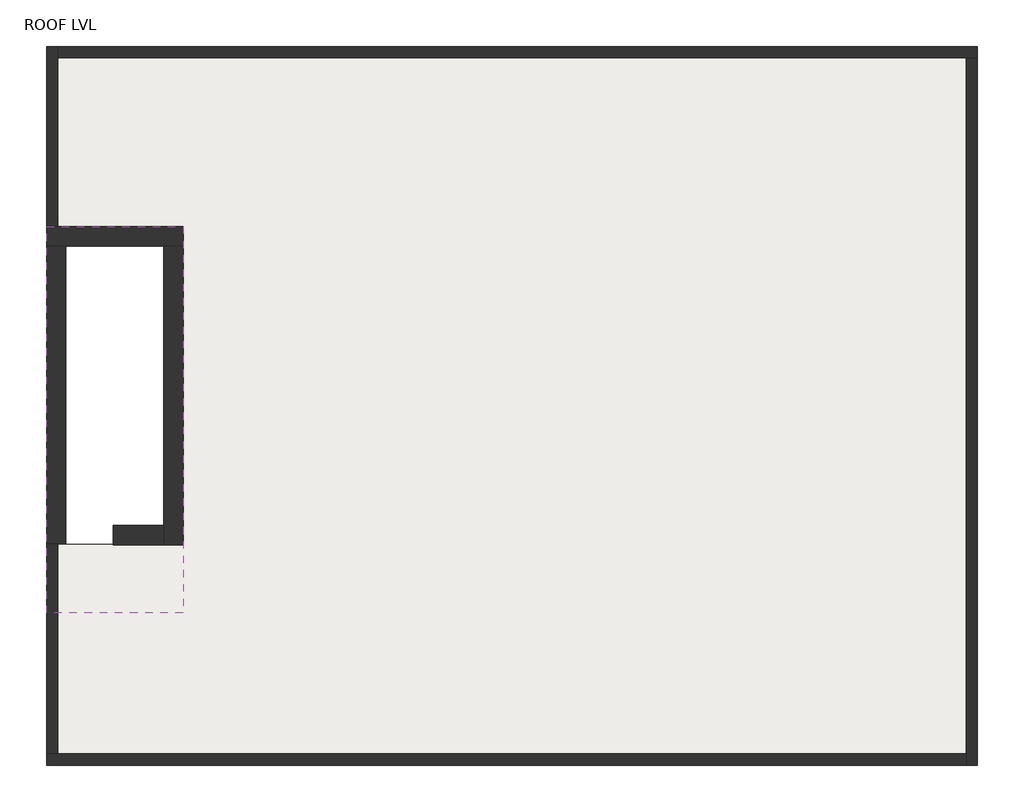
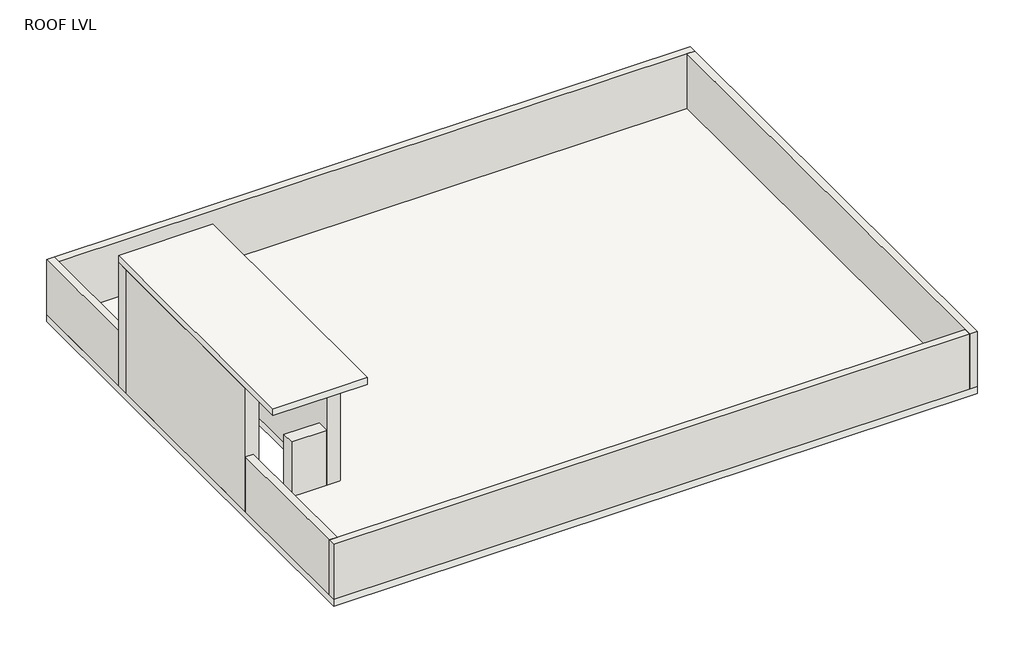
# One storey: 9 walls, 2 slabs.
"""IFC4 building model written with IfcOpenShell, lengths in millimetres."""

from ifc_helpers import new_model, si_unit, frame, origin, place, context, project, spatial, polyline, outline, extrude, faceted_brep, element, save

model = new_model("IFC4")

# Units and contexts
model_context = context("Model", 3, world=origin())
ifc_project = project(units=[si_unit("LENGTHUNIT", "METRE", prefix="MILLI")], contexts=[model_context])

# Site, building, storey
site = spatial("IfcSite", under=ifc_project)
building = spatial("IfcBuilding", under=site)
storey = spatial("IfcBuildingStorey", under=building, Name="ROOF LVL", Elevation=10515.6)

# Slabs
placement = place(None, origin())
element("IfcSlab", 1, ObjectType="Generic - 6\"", at=placement, inside=storey, context=model_context, shape_type="SweptSolid", body=[
    extrude(outline(polyline([(6429.6844404, 8915.7076853), (6429.6844404, -1523.6923147), (-7083.1155596, -1523.6923147), (-7083.1155596, 8915.7076853), (6429.6844404, 8915.7076853)]), holes=[polyline([(-5381.3155596, 6020.1076853), (-6803.7155596, 6020.1076853), (-6803.7155596, 1688.3339108), (-5381.3155596, 1688.3339108), (-5381.3155596, 6020.1076853)])]), frame((0.0, 0.0, 10363.2), z_axis=(0.0, 0.0, 1.0), x_axis=(1.0, 0.0, 0.0)), (0.0, 0.0, 1.0), 152.4),
])
element("IfcSlab", 2, ObjectType="Generic - 6\"", at=placement, inside=storey, context=model_context, shape_type="SweptSolid", body=[
    extrude(outline(polyline([(-5101.9155596, 6299.5076853), (-5101.9155596, 686.9695231), (-7083.1155596, 686.9695231), (-7083.1155596, 6299.5076853), (-5101.9155596, 6299.5076853)])), frame((0.0, 0.0, 13258.8), z_axis=(0.0, 0.0, 1.0), x_axis=(1.0, 0.0, 0.0)), (0.0, 0.0, 1.0), 152.4),
])

# Walls
element("IfcWall", 3, ObjectType="4", at=placement, inside=storey, context=model_context, shape_type="Brep", body=[
    faceted_brep([(-7083.1155596, 8915.7076853, 10515.6), (-7083.1155596, 6299.5076853, 10515.6), (-7083.1155596, 6299.5076853, 11734.8), (-7083.1155596, 8915.7076853, 11734.8), (-6918.0155596, 8915.7076853, 10515.6), (-6918.0155596, 8915.7076853, 11734.8), (-6918.0155596, 8750.6076853, 11734.8), (-6918.0155596, 6299.5076853, 11734.8), (-6918.0155596, 6299.5076853, 10515.6), (-6918.0155596, 8750.6076853, 10515.6)], [[[0, 1, 2, 3]], [[4, 5, 6, 7, 8, 9]], [[1, 0, 4, 9, 8]], [[3, 2, 7, 6, 5]], [[2, 1, 8, 7]], [[0, 3, 5, 4]]]),
])
element("IfcWall", 4, ObjectType="4", at=placement, inside=storey, context=model_context, shape_type="Brep", body=[
    faceted_brep([(-6918.0155596, 8750.6076853, 10515.6), (6264.5844404, 8750.6076853, 10515.6), (6429.6844404, 8750.6076853, 10515.6), (6429.6844404, 8750.6076853, 11734.8), (6264.5844404, 8750.6076853, 11734.8), (-6918.0155596, 8750.6076853, 11734.8), (-6918.0155596, 8915.7076853, 10515.6), (-6918.0155596, 8915.7076853, 11734.8), (6429.6844404, 8915.7076853, 11734.8), (6429.6844404, 8915.7076853, 10515.6)], [[[0, 1, 2, 3, 4, 5]], [[6, 7, 8, 9]], [[2, 1, 0, 6, 9]], [[5, 4, 3, 8, 7]], [[0, 5, 7, 6]], [[3, 2, 9, 8]]]),
])
element("IfcWall", 5, ObjectType="4", at=placement, inside=storey, context=model_context, shape_type="Brep", body=[
    faceted_brep([(6264.5844404, 8750.6076853, 10515.6), (6264.5844404, -1358.5923147, 10515.6), (6264.5844404, -1523.6923147, 10515.6), (6264.5844404, -1523.6923147, 11734.8), (6264.5844404, -1358.5923147, 11734.8), (6264.5844404, 8750.6076853, 11734.8), (6429.6844404, 8750.6076853, 10515.6), (6429.6844404, 8750.6076853, 11734.8), (6429.6844404, -1523.6923147, 11734.8), (6429.6844404, -1523.6923147, 10515.6)], [[[0, 1, 2, 3, 4, 5]], [[6, 7, 8, 9]], [[2, 1, 0, 6, 9]], [[5, 4, 3, 8, 7]], [[0, 5, 7, 6]], [[3, 2, 9, 8]]]),
])
element("IfcWall", 6, ObjectType="4", at=placement, inside=storey, context=model_context, shape_type="Brep", body=[
    faceted_brep([(6264.5844404, -1358.5923147, 10515.6), (-6918.0155596, -1358.5923147, 10515.6), (-7083.1155596, -1358.5923147, 10515.6), (-7083.1155596, -1358.5923147, 11734.8), (-6918.0155596, -1358.5923147, 11734.8), (6264.5844404, -1358.5923147, 11734.8), (6264.5844404, -1523.6923147, 10515.6), (6264.5844404, -1523.6923147, 11734.8), (-7083.1155596, -1523.6923147, 11734.8), (-7083.1155596, -1523.6923147, 10515.6)], [[[0, 1, 2, 3, 4, 5]], [[6, 7, 8, 9]], [[2, 1, 0, 6, 9]], [[5, 4, 3, 8, 7]], [[0, 5, 7, 6]], [[3, 2, 9, 8]]]),
])
element("IfcWall", 7, ObjectType="4", at=placement, inside=storey, context=model_context, shape_type="SweptSolid", body=[
    extrude(outline(polyline([(-6918.0155596, 1688.3339108), (-6918.0155596, -1358.5923147), (-7083.1155596, -1358.5923147), (-7083.1155596, 1688.3339108), (-6918.0155596, 1688.3339108)])), frame((0.0, 0.0, 10515.6), z_axis=(0.0, 0.0, 1.0), x_axis=(1.0, 0.0, 0.0)), (0.0, 0.0, 1.0), 1219.2),
])
element("IfcWall", 8, ObjectType="9", at=placement, inside=storey, context=model_context, shape_type="Brep", body=[
    faceted_brep([(-7083.1155596, 6020.1076853, 13258.8), (-7083.1155596, 6020.1076853, 10515.6), (-6803.7155596, 6020.1076853, 10515.6), (-5381.3155596, 6020.1076853, 10515.6), (-5101.9155596, 6020.1076853, 10515.6), (-5101.9155596, 6020.1076853, 13258.8), (-5381.3155596, 6020.1076853, 13258.8), (-6803.7155596, 6020.1076853, 13258.8), (-7083.1155596, 6299.5076853, 10515.6), (-7083.1155596, 6299.5076853, 11734.8), (-7083.1155596, 6299.5076853, 13258.8), (-5101.9155596, 6299.5076853, 13258.8), (-5101.9155596, 6299.5076853, 10515.6), (-6918.0155596, 6299.5076853, 10515.6)], [[[0, 1, 2, 3, 4, 5, 6, 7]], [[8, 9, 10, 11, 12, 13]], [[4, 3, 2, 1, 8, 13, 12]], [[0, 7, 6, 5, 11, 10]], [[5, 4, 12, 11]], [[0, 10, 9, 8, 1]]]),
])
element("IfcWall", 9, ObjectType="9", at=placement, inside=storey, context=model_context, shape_type="Brep", body=[
    faceted_brep([(-5381.3155596, 6020.1076853, 10515.6), (-5381.3155596, 1956.1076853, 10515.6), (-5381.3155596, 1676.7076853, 10515.6), (-5381.3155596, 1676.7076853, 11734.8), (-5381.3155596, 1676.7076853, 13258.8), (-5381.3155596, 6020.1076853, 13258.8), (-5101.9155596, 6020.1076853, 10515.6), (-5101.9155596, 6020.1076853, 13258.8), (-5101.9155596, 1676.7076853, 13258.8), (-5101.9155596, 1676.7076853, 10515.6)], [[[0, 1, 2, 3, 4, 5]], [[6, 7, 8, 9]], [[2, 1, 0, 6, 9]], [[5, 4, 8, 7]], [[0, 5, 7, 6]], [[4, 3, 2, 9, 8]]]),
])
element("IfcWall", 10, ObjectType="9", at=placement, inside=storey, context=model_context, shape_type="SweptSolid", body=[
    extrude(outline(polyline([(-6117.9155596, 1956.1076853), (-5381.3155596, 1956.1076853), (-5381.3155596, 1676.7076853), (-6117.9155596, 1676.7076853), (-6117.9155596, 1956.1076853)])), frame((0.0, 0.0, 10515.6), z_axis=(0.0, 0.0, 1.0), x_axis=(1.0, 0.0, 0.0)), (0.0, 0.0, 1.0), 1219.2),
])
element("IfcWall", 11, ObjectType="9", at=placement, inside=storey, context=model_context, shape_type="Brep", body=[
    faceted_brep([(-6803.7155596, 1688.3339108, 10515.6), (-6803.7155596, 6020.1076853, 10515.6), (-6803.7155596, 6020.1076853, 13258.8), (-6803.7155596, 1688.3339108, 13258.8), (-7083.1155596, 1688.3339108, 10515.6), (-7083.1155596, 1688.3339108, 11734.8), (-7083.1155596, 1688.3339108, 13258.8), (-7083.1155596, 6020.1076853, 13258.8), (-7083.1155596, 6020.1076853, 10515.6), (-6918.0155596, 1688.3339108, 10515.6)], [[[0, 1, 2, 3]], [[4, 5, 6, 7, 8]], [[1, 0, 9, 4, 8]], [[3, 2, 7, 6]], [[0, 3, 6, 5, 4, 9]], [[1, 8, 7, 2]]]),
])

save(model, "model.ifc")

# Revit data of these elements
# Type "Generic - 6\""
#   Assembly Code = "B1010"
#   Function = 0
#   Layers, outside or top first: 0' - 6" no material (function 1)
# Type "4"
#   Assembly Code = "B2010"
#   Layers, outside or top first: 0' - 1" "Gypsum Wall Board" (function 1); 0' - 4 1/2" no material (function 1); 0' - 1" "Gypsum Wall Board" (function 1)
# Type "9"
#   Assembly Code = "B2010"
#   Layers, outside or top first: 0' - 1" "Gypsum Wall Board" (function 1); 0' - 9" no material (function 1); 0' - 1" "Gypsum Wall Board" (function 1)
# Element 1 (IfcSlab, "Generic - 6\"")
#   Height Offset From Level = 0' - 0"
#   Phase Created = New Construction
#   Materials on its faces: "Default Floor"
# Element 2 (IfcSlab, "Generic - 6\"")
#   Height Offset From Level = 9' - 6"
#   Phase Created = New Construction
#   Materials on its faces: "Default Floor"
# Elements 3, 4, 5, 6 (IfcWall, "4")
#   Top Offset = 0' - 0"
#   Base Offset = 0' - 0"
#   wall height = 4' - 0"
#   Phase Created = New Construction
#   Base Constraint = ROOF LVL
#   Top Constraint = PARAPET WALL LVL
#   Materials on its faces: "Gypsum Wall Board", "Default Wall"
# Element 7 (IfcWall, "4")
#   Top Offset = 0' - 0"
#   Base Offset = 0' - 0"
#   wall height = 4' - 0"
#   Phase Created = New Construction
#   Base Constraint = ROOF LVL
#   Top Constraint = PARAPET WALL LVL
#   Materials on its faces: "Default Wall", "Gypsum Wall Board"
# Elements 8, 9 (IfcWall, "9")
#   Top Offset = 0' - 0"
#   Base Offset = 0' - 0"
#   Unconnected Height = 9' - 0"
#   wall height = 9' - 0"
#   Phase Created = New Construction
#   Base Constraint = ROOF LVL
#   Materials on its faces: "Gypsum Wall Board", "Default Wall"
# Element 10 (IfcWall, "9")
#   Top Offset = 0' - 0"
#   Base Offset = 0' - 0"
#   Unconnected Height = 4' - 0"
#   wall height = 4' - 0"
#   Phase Created = New Construction
#   Base Constraint = ROOF LVL
#   Materials on its faces: "Default Wall", "Gypsum Wall Board"
# Element 11 (IfcWall, "9")
#   Top Offset = 0' - 0"
#   Base Offset = 0' - 0"
#   Unconnected Height = 9' - 0"
#   wall height = 9' - 0"
#   Phase Created = New Construction
#   Base Constraint = ROOF LVL
#   Materials on its faces: "Default Wall", "Gypsum Wall Board"
# Materials
#   "Gypsum Wall Board": class "Generic", colour RGB 228 228 228, transparency 0, Description = "Gypsum Wall Board", Cost = 0
#   "Default Floor": colour RGB 128 128 128, transparency 0, Cost = 0
#   "Default Wall": colour RGB 128 128 128, transparency 0, Cost = 0
